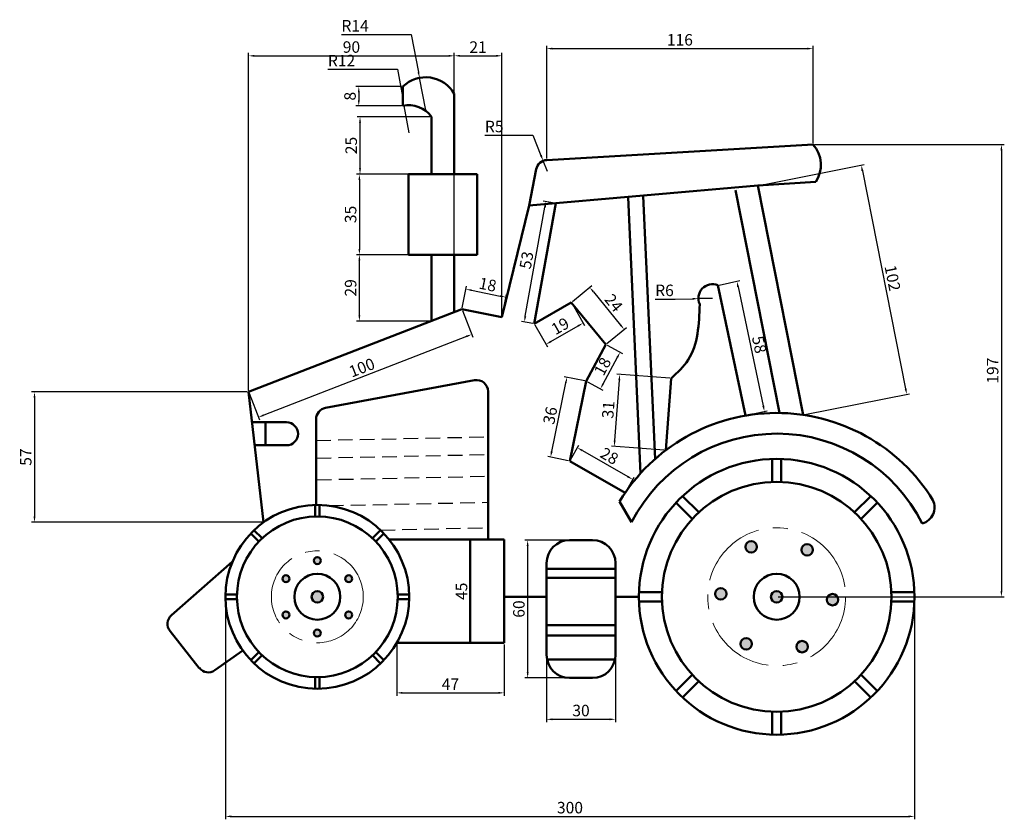
# Model space of a CAD drawing. Units: millimetres. Extents: x 853 to 1282, y 1256 to 1604.
import ezdxf

# ---------------------------------------------------------------- set-up
doc = ezdxf.new("R2010")
doc.units = ezdxf.units.MM
doc.linetypes.add('CENTER', pattern=[50.8, 31.75, -6.35, 6.35, -6.35])
doc.linetypes.add('HIDDEN', pattern=[9.525, 6.35, -3.175])
for name, color, linetype, lineweight in [('M-CNTR', 1, 'CENTER', 18), ('M-DIMS', 2, 'Continuous', 25), ('M-HATC', 8, 'Continuous', 18), ('M-HIDN', 8, 'HIDDEN', 25), ('M-OUTL', 7, 'Continuous', 50)]:
    doc.layers.add(name, color=color, linetype=linetype, lineweight=lineweight)
doc.styles.get("Standard").update_dxf_attribs({"font": 'arial.ttf'})
doc.dimstyles.new('ISO-25', dxfattribs={"dimtxt": 5, "dimasz": 2.5, "dimexe": 1.25, "dimexo": 0.625, "dimtad": 1, "dimtoh": 1, "dimdec": 0, "dimtxsty": 'Standard', "dimcen": 2.5, "dimadec": 0, "dimazin": 0, "dimtfac": 1, "dimtdec": 0, "dimtmove": 0, "dimatfit": 3, "dimfxl": 1, "dimarcsym": 0})

# ---------------------------------------------------------------- blocks, each defined once
blk = doc.blocks.new('*U1')
for p, q in [((-1, 2.5), (-1, -2.5)), ((1, 2.5), (1, -2.5))]:
    blk.add_line(p, q)
blk = doc.blocks.new('*U2')
at = {"layer": 'M-OUTL', "color": 0, "linetype": 'ByBlock', "lineweight": -2, "transparency": 16777216}
blk.add_blockref('*U1', (982.95, 1390.56), dxfattribs=at)
for p, rotation in [((956.43, 1379.58), 45.00000000000001), ((1009.46, 1379.58), 315), ((945.45, 1353.06), 90), ((1020.45, 1353.06), 270), ((956.43, 1326.55), 135), ((1009.46, 1326.55), 225), ((982.95, 1315.56), 180)]:
    blk.add_blockref('*U1', p, dxfattribs=dict(at, rotation=rotation))
blk = doc.blocks.new('*U3')
for p, q in [((-2, -5), (-2, 5)), ((2, -5), (2, 5))]:
    blk.add_line(p, q)
blk = doc.blocks.new('*U4')
at = {"layer": 'M-OUTL', "color": 0, "linetype": 'ByBlock', "lineweight": -2, "transparency": 16777216}
blk.add_blockref('*U3', (1182.95, 1408.06), dxfattribs=at)
for p, rotation in [((1144.05, 1391.96), 45.00000000000001), ((1221.84, 1391.96), 315.0000000000001), ((1127.95, 1353.06), 90), ((1237.95, 1353.06), 270.0000000000001), ((1144.05, 1314.17), 135), ((1221.84, 1314.17), 225), ((1182.95, 1298.06), 180)]:
    blk.add_blockref('*U3', p, dxfattribs=dict(at, rotation=rotation))
blk = doc.blocks.new('*U5')
blk.add_circle((0, 0), 1.5)
blk = doc.blocks.new('*U6')
at = {"layer": 'M-OUTL', "color": 0, "linetype": 'ByBlock', "lineweight": -2, "transparency": 16777216}
blk.add_blockref('*U5', (982.95, 1368.83), dxfattribs=at)
for p, rotation in [((969.3, 1360.95), 60), ((996.6, 1360.94), 300), ((969.3, 1345.19), 120), ((996.59, 1345.18), 240), ((982.94, 1337.3), 180)]:
    blk.add_blockref('*U5', p, dxfattribs=dict(at, rotation=rotation))
blk = doc.blocks.new('*U7')
blk.add_circle((0, 0), 2.5)
blk = doc.blocks.new('*U8')
at = {"layer": 'M-OUTL', "color": 0, "linetype": 'ByBlock', "lineweight": -2, "transparency": 16777216}
for p, rotation in [((1171.87, 1374.78), 59.99999999999999), ((1158.6, 1354.33), 120), ((1207.29, 1351.8), 300), ((1169.68, 1332.61), 180), ((1194.02, 1331.35), 239.9999999999999)]:
    blk.add_blockref('*U7', p, dxfattribs=dict(at, rotation=rotation))
blk.add_blockref('*U7', (1196.21, 1373.52), dxfattribs=at)
blk = doc.blocks.new('*D9')
at = {"layer": 'Defpoints', "color": 0, "lineweight": 100, "transparency": 16777216}
for p in [(942.95, 1353.06), (1242.95, 1353.06), (1242.95, 1257.5)]:
    blk.add_point(p, dxfattribs=at)
at = {"layer": 'M-DIMS', "color": 0, "lineweight": -2, "transparency": 16777216}
for p, q in [((942.95, 1352.44), (942.95, 1256.25)), ((1242.95, 1352.44), (1242.95, 1256.25)), ((945.45, 1257.5), (1240.45, 1257.5))]:
    blk.add_line(p, q, dxfattribs=at)
at = {"layer": 'M-DIMS', "color": 0, "lineweight": 100, "transparency": 16777216}
for points in [[(945.45, 1257.91), (945.45, 1257.08), (942.95, 1257.5)], [(1240.45, 1257.91), (1240.45, 1257.08), (1242.95, 1257.5)]]:
    blk.add_solid(points, dxfattribs=at)
at = {"layer": 'M-DIMS', "color": 0, "transparency": 16777216, "insert": (1092.95, 1260.67), "char_height": 5, "attachment_point": 5}
blk.add_mtext('300', dxfattribs=at)
blk = doc.blocks.new('*D10')
at = {"layer": 'Defpoints', "color": 0, "lineweight": 100, "transparency": 16777216}
for p in [(1198.77, 1549.9), (1182.95, 1353.06), (1280.81, 1353.06)]:
    blk.add_point(p, dxfattribs=at)
at = {"layer": 'M-DIMS', "color": 0, "lineweight": -2, "transparency": 16777216}
for p, q in [((1199.39, 1549.9), (1282.06, 1549.9)), ((1280.81, 1547.4), (1280.81, 1355.56)), ((1183.57, 1353.06), (1282.06, 1353.06))]:
    blk.add_line(p, q, dxfattribs=at)
at = {"layer": 'M-DIMS', "color": 0, "lineweight": 100, "transparency": 16777216}
for points in [[(1280.4, 1547.4), (1281.23, 1547.4), (1280.81, 1549.9)], [(1280.4, 1355.56), (1281.23, 1355.56), (1280.81, 1353.06)]]:
    blk.add_solid(points, dxfattribs=at)
at = {"layer": 'M-DIMS', "color": 0, "transparency": 16777216, "insert": (1277.64, 1451.48), "char_height": 5, "attachment_point": 5, "rotation": 90}
blk.add_mtext('197', dxfattribs=at)
blk = doc.blocks.new('*D11')
at = {"layer": 'Defpoints', "color": 0, "lineweight": 100, "transparency": 16777216}
for p in [(953.02, 1442.19), (859.8, 1385.51), (959.55, 1385.51)]:
    blk.add_point(p, dxfattribs=at)
at = {"layer": 'M-DIMS', "color": 0, "lineweight": -2, "transparency": 16777216}
for p, q in [((952.4, 1442.19), (858.55, 1442.19)), ((859.8, 1439.69), (859.8, 1388.01)), ((958.92, 1385.51), (858.55, 1385.51))]:
    blk.add_line(p, q, dxfattribs=at)
at = {"layer": 'M-DIMS', "color": 0, "lineweight": 100, "transparency": 16777216}
for points in [[(859.39, 1439.69), (860.22, 1439.69), (859.8, 1442.19)], [(859.39, 1388.01), (860.22, 1388.01), (859.8, 1385.51)]]:
    blk.add_solid(points, dxfattribs=at)
at = {"layer": 'M-DIMS', "color": 0, "transparency": 16777216, "insert": (856.64, 1413.85), "char_height": 5, "attachment_point": 5, "rotation": 90}
blk.add_mtext('57', dxfattribs=at)
blk = doc.blocks.new('*D12')
at = {"layer": 'Defpoints', "color": 0, "lineweight": 100, "transparency": 16777216}
for p in [(1042.59, 1588.46), (1042.59, 1476.94), (953.02, 1442.19)]:
    blk.add_point(p, dxfattribs=at)
at = {"layer": 'M-DIMS', "color": 0, "lineweight": -2, "transparency": 16777216}
for p, q in [((953.02, 1442.81), (953.02, 1589.71)), ((955.52, 1588.46), (1040.09, 1588.46)), ((1042.59, 1477.57), (1042.59, 1589.71))]:
    blk.add_line(p, q, dxfattribs=at)
at = {"layer": 'M-DIMS', "color": 0, "lineweight": 100, "transparency": 16777216}
for points in [[(955.52, 1588.87), (955.52, 1588.04), (953.02, 1588.46)], [(1040.09, 1588.87), (1040.09, 1588.04), (1042.59, 1588.46)]]:
    blk.add_solid(points, dxfattribs=at)
at = {"layer": 'M-DIMS', "color": 0, "transparency": 16777216, "insert": (997.8, 1591.64), "char_height": 5, "attachment_point": 5}
blk.add_mtext('90', dxfattribs=at)
blk = doc.blocks.new('*D13')
at = {"layer": 'Defpoints', "color": 0, "lineweight": 100, "transparency": 16777216}
for p in [(1198.77, 1591.61), (1198.77, 1549.9), (1082.84, 1543.13)]:
    blk.add_point(p, dxfattribs=at)
at = {"layer": 'M-DIMS', "color": 0, "lineweight": -2, "transparency": 16777216}
for p, q in [((1082.84, 1543.75), (1082.84, 1592.86)), ((1085.34, 1591.61), (1196.27, 1591.61)), ((1198.77, 1550.52), (1198.77, 1592.86))]:
    blk.add_line(p, q, dxfattribs=at)
at = {"layer": 'M-DIMS', "color": 0, "lineweight": 100, "transparency": 16777216}
for points in [[(1085.34, 1592.03), (1085.34, 1591.19), (1082.84, 1591.61)], [(1196.27, 1592.03), (1196.27, 1591.19), (1198.77, 1591.61)]]:
    blk.add_solid(points, dxfattribs=at)
at = {"layer": 'M-DIMS', "color": 0, "transparency": 16777216, "insert": (1140.8, 1594.79), "char_height": 5, "attachment_point": 5}
blk.add_mtext('116', dxfattribs=at)
blk = doc.blocks.new('*D14')
at = {"layer": 'Defpoints', "color": 0, "lineweight": 100, "transparency": 16777216}
for p in [(1063.29, 1588.49), (1042.59, 1476.94), (1063.29, 1474.7)]:
    blk.add_point(p, dxfattribs=at)
at = {"layer": 'M-DIMS', "color": 0, "lineweight": -2, "transparency": 16777216}
for p, q in [((1042.59, 1477.57), (1042.59, 1589.74)), ((1045.09, 1588.49), (1060.79, 1588.49)), ((1063.29, 1475.32), (1063.29, 1589.74))]:
    blk.add_line(p, q, dxfattribs=at)
at = {"layer": 'M-DIMS', "color": 0, "lineweight": 100, "transparency": 16777216}
for points in [[(1045.09, 1588.9), (1045.09, 1588.07), (1042.59, 1588.49)], [(1060.79, 1588.9), (1060.79, 1588.07), (1063.29, 1588.49)]]:
    blk.add_solid(points, dxfattribs=at)
at = {"layer": 'M-DIMS', "color": 0, "transparency": 16777216, "insert": (1052.94, 1591.62), "char_height": 5, "attachment_point": 5}
blk.add_mtext('21', dxfattribs=at)
blk = doc.blocks.new('*D15')
at = {"layer": 'Defpoints', "color": 0, "lineweight": 100, "transparency": 16777216}
for p in [(1082.76, 1347.74), (1112.76, 1347.74), (1112.76, 1299.75)]:
    blk.add_point(p, dxfattribs=at)
at = {"layer": 'M-DIMS', "color": 0, "lineweight": -2, "transparency": 16777216}
for p, q in [((1082.76, 1347.12), (1082.76, 1298.5)), ((1112.76, 1347.12), (1112.76, 1298.5)), ((1085.26, 1299.75), (1110.26, 1299.75))]:
    blk.add_line(p, q, dxfattribs=at)
at = {"layer": 'M-DIMS', "color": 0, "lineweight": 100, "transparency": 16777216}
for points in [[(1085.26, 1300.16), (1085.26, 1299.33), (1082.76, 1299.75)], [(1110.26, 1300.16), (1110.26, 1299.33), (1112.76, 1299.75)]]:
    blk.add_solid(points, dxfattribs=at)
at = {"layer": 'M-DIMS', "color": 0, "transparency": 16777216, "insert": (1097.76, 1302.93), "char_height": 5, "attachment_point": 5}
blk.add_mtext('30', dxfattribs=at)
blk = doc.blocks.new('*D16')
at = {"layer": 'Defpoints', "color": 0, "lineweight": 100, "transparency": 16777216}
for p in [(1097.76, 1377.74), (1074.52, 1317.74), (1097.76, 1317.74)]:
    blk.add_point(p, dxfattribs=at)
at = {"layer": 'M-DIMS', "color": 0, "lineweight": -2, "transparency": 16777216}
for p, q in [((1097.14, 1377.74), (1073.27, 1377.74)), ((1074.52, 1375.24), (1074.52, 1320.24)), ((1097.14, 1317.74), (1073.27, 1317.74))]:
    blk.add_line(p, q, dxfattribs=at)
at = {"layer": 'M-DIMS', "color": 0, "lineweight": 100, "transparency": 16777216}
for points in [[(1074.11, 1375.24), (1074.94, 1375.24), (1074.52, 1377.74)], [(1074.11, 1320.24), (1074.94, 1320.24), (1074.52, 1317.74)]]:
    blk.add_solid(points, dxfattribs=at)
at = {"layer": 'M-DIMS', "color": 0, "transparency": 16777216, "insert": (1071.35, 1347.74), "char_height": 5, "attachment_point": 5, "rotation": 90}
blk.add_mtext('60', dxfattribs=at)
blk = doc.blocks.new('*D17')
at = {"layer": 'Defpoints', "color": 0, "lineweight": 100, "transparency": 16777216}
for p in [(1049.53, 1377.96), (1049.53, 1332.96), (1049.53, 1332.96)]:
    blk.add_point(p, dxfattribs=at)
at = {"layer": 'M-DIMS', "color": 0, "lineweight": -2, "transparency": 16777216}
for p, q in [((1050.16, 1377.96), (1050.78, 1377.96)), ((1049.53, 1375.46), (1049.53, 1335.46)), ((1050.16, 1332.96), (1050.78, 1332.96))]:
    blk.add_line(p, q, dxfattribs=at)
at = {"layer": 'M-DIMS', "color": 0, "lineweight": 100, "transparency": 16777216}
for points in [[(1049.12, 1375.46), (1049.95, 1375.46), (1049.53, 1377.96)], [(1049.12, 1335.46), (1049.95, 1335.46), (1049.53, 1332.96)]]:
    blk.add_solid(points, dxfattribs=at)
at = {"layer": 'M-DIMS', "color": 0, "transparency": 16777216, "insert": (1046.37, 1355.46), "char_height": 5, "attachment_point": 5, "rotation": 90}
blk.add_mtext('45', dxfattribs=at)
blk = doc.blocks.new('*D18')
at = {"layer": 'Defpoints', "color": 0, "lineweight": 100, "transparency": 16777216}
for p in [(1017.53, 1332.96), (1064.25, 1332.96), (1064.25, 1311.26)]:
    blk.add_point(p, dxfattribs=at)
at = {"layer": 'M-DIMS', "color": 0, "lineweight": -2, "transparency": 16777216}
for p, q in [((1017.53, 1332.33), (1017.53, 1310.01)), ((1064.25, 1332.33), (1064.25, 1310.01)), ((1020.03, 1311.26), (1061.75, 1311.26))]:
    blk.add_line(p, q, dxfattribs=at)
at = {"layer": 'M-DIMS', "color": 0, "lineweight": 100, "transparency": 16777216}
for points in [[(1020.03, 1311.68), (1020.03, 1310.84), (1017.53, 1311.26)], [(1061.75, 1311.68), (1061.75, 1310.84), (1064.25, 1311.26)]]:
    blk.add_solid(points, dxfattribs=at)
at = {"layer": 'M-DIMS', "color": 0, "transparency": 16777216, "insert": (1040.89, 1314.38), "char_height": 5, "attachment_point": 5}
blk.add_mtext('47', dxfattribs=at)
blk = doc.blocks.new('*D19')
at = {"layer": 'Defpoints', "color": 0, "lineweight": 100, "transparency": 16777216}
for p in [(1174.77, 1531.97), (1239.58, 1441.15), (1194.55, 1432.22)]:
    blk.add_point(p, dxfattribs=at)
at = {"layer": 'M-DIMS', "color": 0, "lineweight": -2, "transparency": 16777216}
for p, q in [((1175.38, 1532.09), (1221.02, 1541.14)), ((1220.28, 1538.45), (1239.09, 1443.6)), ((1195.16, 1432.34), (1240.8, 1441.39))]:
    blk.add_line(p, q, dxfattribs=at)
at = {"layer": 'M-DIMS', "color": 0, "lineweight": 100, "transparency": 16777216}
for points in [[(1220.69, 1538.53), (1219.87, 1538.37), (1219.8, 1540.9)], [(1239.5, 1443.68), (1238.68, 1443.52), (1239.58, 1441.15)]]:
    blk.add_solid(points, dxfattribs=at)
at = {"layer": 'M-DIMS', "color": 0, "transparency": 16777216, "insert": (1232.8, 1491.64), "char_height": 5, "attachment_point": 5, "rotation": 281.2154}
blk.add_mtext('102', dxfattribs=at)
blk = doc.blocks.new('*D20')
at = {"layer": 'Defpoints', "color": 0, "lineweight": 100, "transparency": 16777216}
for p in [(1157.31, 1488.61), (1169.34, 1431.9), (1177.65, 1433.66)]:
    blk.add_point(p, dxfattribs=at)
at = {"layer": 'M-DIMS', "color": 0, "lineweight": -2, "transparency": 16777216}
for p, q in [((1157.92, 1488.74), (1166.84, 1490.63)), ((1166.14, 1487.93), (1177.13, 1436.11)), ((1169.95, 1432.03), (1178.87, 1433.92))]:
    blk.add_line(p, q, dxfattribs=at)
at = {"layer": 'M-DIMS', "color": 0, "lineweight": 100, "transparency": 16777216}
for points in [[(1166.55, 1488.02), (1165.73, 1487.84), (1165.62, 1490.37)], [(1177.54, 1436.19), (1176.72, 1436.02), (1177.65, 1433.66)]]:
    blk.add_solid(points, dxfattribs=at)
at = {"layer": 'M-DIMS', "color": 0, "transparency": 16777216, "insert": (1174.74, 1462.68), "char_height": 5, "attachment_point": 5, "rotation": 281.9736}
blk.add_mtext('58', dxfattribs=at)
blk = doc.blocks.new('*D21')
at = {"layer": 'Defpoints', "color": 0, "lineweight": 100, "transparency": 16777216}
for p in [(1137.03, 1448.09), (1112.22, 1418.55), (1134.64, 1416.83)]:
    blk.add_point(p, dxfattribs=at)
at = {"layer": 'M-DIMS', "color": 0, "lineweight": -2, "transparency": 16777216}
for p, q in [((1136.41, 1448.13), (1113.37, 1449.9)), ((1114.42, 1447.31), (1112.41, 1421.04)), ((1134.02, 1416.88), (1110.98, 1418.65))]:
    blk.add_line(p, q, dxfattribs=at)
at = {"layer": 'M-DIMS', "color": 0, "lineweight": 100, "transparency": 16777216}
for points in [[(1114.01, 1447.34), (1114.84, 1447.28), (1114.61, 1449.8)], [(1112, 1421.07), (1112.83, 1421.01), (1112.22, 1418.55)]]:
    blk.add_solid(points, dxfattribs=at)
at = {"layer": 'M-DIMS', "color": 0, "transparency": 16777216, "insert": (1110.25, 1434.42), "char_height": 5, "attachment_point": 5, "rotation": 85.6221}
blk.add_mtext('31', dxfattribs=at)
blk = doc.blocks.new('*D22')
at = {"layer": 'Defpoints', "color": 0, "lineweight": 100, "transparency": 16777216}
for p in [(1092.82, 1412.09), (1120.29, 1404.11), (1116.94, 1398.26)]:
    blk.add_point(p, dxfattribs=at)
at = {"layer": 'M-DIMS', "color": 0, "lineweight": -2, "transparency": 16777216}
for p, q in [((1093.13, 1412.64), (1096.8, 1419.02)), ((1098.35, 1416.7), (1118.12, 1405.35)), ((1117.25, 1398.8), (1120.91, 1405.19))]:
    blk.add_line(p, q, dxfattribs=at)
at = {"layer": 'M-DIMS', "color": 0, "lineweight": 100, "transparency": 16777216}
for points in [[(1098.55, 1417.06), (1098.14, 1416.33), (1096.18, 1417.94)], [(1118.33, 1405.71), (1117.91, 1404.99), (1120.29, 1404.11)]]:
    blk.add_solid(points, dxfattribs=at)
at = {"layer": 'M-DIMS', "color": 0, "transparency": 16777216, "insert": (1109.81, 1413.78), "char_height": 5, "attachment_point": 5, "rotation": 330.159}
blk.add_mtext('28', dxfattribs=at)
blk = doc.blocks.new('*D23')
at = {"layer": 'Defpoints', "color": 0, "lineweight": 100, "transparency": 16777216}
for p in [(1091.65, 1448.59), (1099.98, 1446.87), (1092.82, 1412.09)]:
    blk.add_point(p, dxfattribs=at)
at = {"layer": 'M-DIMS', "color": 0, "lineweight": -2, "transparency": 16777216}
for p, q in [((1085, 1416.26), (1091.14, 1446.14)), ((1099.36, 1447), (1090.42, 1448.84)), ((1092.21, 1412.22), (1083.27, 1414.06))]:
    blk.add_line(p, q, dxfattribs=at)
at = {"layer": 'M-DIMS', "color": 0, "lineweight": 100, "transparency": 16777216}
for points in [[(1090.74, 1446.22), (1091.55, 1446.05), (1091.65, 1448.59)], [(1084.59, 1416.34), (1085.41, 1416.17), (1084.5, 1413.81)]]:
    blk.add_solid(points, dxfattribs=at)
at = {"layer": 'M-DIMS', "color": 0, "transparency": 16777216, "insert": (1084.96, 1431.84), "char_height": 5, "attachment_point": 5, "rotation": 78.3786}
blk.add_mtext('36', dxfattribs=at)
blk = doc.blocks.new('*D24')
at = {"layer": 'Defpoints', "color": 0, "lineweight": 100, "transparency": 16777216}
for p in [(1108.56, 1462.83), (1114.78, 1459.49), (1099.98, 1446.87)]:
    blk.add_point(p, dxfattribs=at)
at = {"layer": 'M-DIMS', "color": 0, "lineweight": -2, "transparency": 16777216}
for p, q in [((1109.11, 1462.54), (1115.89, 1458.89)), ((1107.39, 1445.73), (1113.6, 1457.28)), ((1100.53, 1446.58), (1107.3, 1442.93))]:
    blk.add_line(p, q, dxfattribs=at)
at = {"layer": 'M-DIMS', "color": 0, "lineweight": 100, "transparency": 16777216}
for points in [[(1113.23, 1457.48), (1113.97, 1457.09), (1114.78, 1459.49)], [(1107.02, 1445.92), (1107.75, 1445.53), (1106.2, 1443.53)]]:
    blk.add_solid(points, dxfattribs=at)
at = {"layer": 'M-DIMS', "color": 0, "transparency": 16777216, "insert": (1107.69, 1453.01), "char_height": 5, "attachment_point": 5, "rotation": 61.7294}
blk.add_mtext('18', dxfattribs=at)
blk = doc.blocks.new('*D25')
at = {"layer": 'Defpoints', "color": 0, "lineweight": 100, "transparency": 16777216}
for p in [(1093.54, 1481.18), (1116.57, 1469.4), (1108.56, 1462.83)]:
    blk.add_point(p, dxfattribs=at)
at = {"layer": 'M-DIMS', "color": 0, "lineweight": -2, "transparency": 16777216}
for p, q in [((1094.02, 1481.57), (1102.52, 1488.53)), ((1103.14, 1485.8), (1114.99, 1471.33)), ((1109.04, 1463.23), (1117.54, 1470.19))]:
    blk.add_line(p, q, dxfattribs=at)
at = {"layer": 'M-DIMS', "color": 0, "lineweight": 100, "transparency": 16777216}
for points in [[(1103.46, 1486.07), (1102.81, 1485.54), (1101.55, 1487.74)], [(1115.31, 1471.59), (1114.67, 1471.07), (1116.57, 1469.4)]]:
    blk.add_solid(points, dxfattribs=at)
at = {"layer": 'M-DIMS', "color": 0, "transparency": 16777216, "insert": (1111.49, 1480.55), "char_height": 5, "attachment_point": 5, "rotation": 309.3139}
blk.add_mtext('24', dxfattribs=at)
blk = doc.blocks.new('*D26')
at = {"layer": 'Defpoints', "color": 0, "lineweight": 100, "transparency": 16777216}
for p in [(1093.54, 1481.18), (1077.33, 1471.89), (1098.69, 1472.19)]:
    blk.add_point(p, dxfattribs=at)
at = {"layer": 'M-DIMS', "color": 0, "lineweight": -2, "transparency": 16777216}
for p, q in [((1093.85, 1480.63), (1099.31, 1471.11)), ((1077.64, 1471.34), (1083.1, 1461.82)), ((1084.64, 1464.15), (1096.52, 1470.95))]:
    blk.add_line(p, q, dxfattribs=at)
at = {"layer": 'M-DIMS', "color": 0, "lineweight": 100, "transparency": 16777216}
for points in [[(1096.31, 1471.31), (1096.72, 1470.59), (1098.69, 1472.19)], [(1084.44, 1464.51), (1084.85, 1463.78), (1082.47, 1462.9)]]:
    blk.add_solid(points, dxfattribs=at)
at = {"layer": 'M-DIMS', "color": 0, "transparency": 16777216, "insert": (1089, 1470.3), "char_height": 5, "attachment_point": 5, "rotation": 29.8139}
blk.add_mtext('19', dxfattribs=at)
blk = doc.blocks.new('*D27')
at = {"layer": 'Defpoints', "color": 0, "lineweight": 100, "transparency": 16777216}
for p in [(1082.52, 1525.06), (1086.78, 1524.29), (1077.33, 1471.89)]:
    blk.add_point(p, dxfattribs=at)
at = {"layer": 'M-DIMS', "color": 0, "lineweight": -2, "transparency": 16777216}
for p, q in [((1073.51, 1475.12), (1082.07, 1522.6)), ((1086.17, 1524.4), (1081.29, 1525.28)), ((1076.71, 1472), (1071.83, 1472.88))]:
    blk.add_line(p, q, dxfattribs=at)
at = {"layer": 'M-DIMS', "color": 0, "lineweight": 100, "transparency": 16777216}
for points in [[(1081.66, 1522.67), (1082.48, 1522.52), (1082.52, 1525.06)], [(1073.1, 1475.19), (1073.92, 1475.04), (1073.06, 1472.65)]]:
    blk.add_solid(points, dxfattribs=at)
at = {"layer": 'M-DIMS', "color": 0, "transparency": 16777216, "insert": (1074.66, 1499.42), "char_height": 5, "attachment_point": 5, "rotation": 79.7728}
blk.add_mtext('53', dxfattribs=at)
blk = doc.blocks.new('*D28')
at = {"layer": 'Defpoints', "color": 0, "lineweight": 100, "transparency": 16777216}
for p in [(1065.06, 1483.42), (1045.92, 1478.23), (1063.29, 1474.7)]:
    blk.add_point(p, dxfattribs=at)
at = {"layer": 'M-DIMS', "color": 0, "lineweight": -2, "transparency": 16777216}
for p, q in [((1046.04, 1478.84), (1047.94, 1488.18)), ((1050.14, 1486.46), (1062.61, 1483.92)), ((1063.41, 1475.31), (1065.31, 1484.65))]:
    blk.add_line(p, q, dxfattribs=at)
at = {"layer": 'M-DIMS', "color": 0, "lineweight": 100, "transparency": 16777216}
for points in [[(1050.23, 1486.87), (1050.06, 1486.05), (1047.69, 1486.96)], [(1062.69, 1484.33), (1062.53, 1483.51), (1065.06, 1483.42)]]:
    blk.add_solid(points, dxfattribs=at)
at = {"layer": 'M-DIMS', "color": 0, "transparency": 16777216, "insert": (1057.01, 1488.3), "char_height": 5, "attachment_point": 5, "rotation": 348.5016}
blk.add_mtext('18', dxfattribs=at)
blk = doc.blocks.new('*D29')
at = {"layer": 'Defpoints', "color": 0, "lineweight": 100, "transparency": 16777216}
for p in [(1045.92, 1478.23), (953.02, 1442.19), (957.28, 1431.21)]:
    blk.add_point(p, dxfattribs=at)
at = {"layer": 'M-DIMS', "color": 0, "lineweight": -2, "transparency": 16777216}
for p, q in [((1046.14, 1477.65), (1050.63, 1466.08)), ((1047.85, 1466.34), (959.61, 1432.11)), ((953.25, 1441.61), (957.73, 1430.04))]:
    blk.add_line(p, q, dxfattribs=at)
at = {"layer": 'M-DIMS', "color": 0, "lineweight": 100, "transparency": 16777216}
for points in [[(1047.7, 1466.73), (1048, 1465.96), (1050.18, 1467.25)], [(959.46, 1432.5), (959.76, 1431.72), (957.28, 1431.21)]]:
    blk.add_solid(points, dxfattribs=at)
at = {"layer": 'M-DIMS', "color": 0, "transparency": 16777216, "insert": (1002.58, 1452.19), "char_height": 5, "attachment_point": 5, "rotation": 21.2055}
blk.add_mtext('100', dxfattribs=at)
blk = doc.blocks.new('*D30')
at = {"layer": 'Defpoints', "color": 0, "lineweight": 100, "transparency": 16777216}
for p in [(1001.26, 1501.94), (1032.59, 1501.94), (1032.59, 1473.06)]:
    blk.add_point(p, dxfattribs=at)
at = {"layer": 'M-DIMS', "color": 0, "lineweight": -2, "transparency": 16777216}
for p, q in [((1031.96, 1501.94), (1000.01, 1501.94)), ((1001.26, 1475.56), (1001.26, 1499.44)), ((1031.96, 1473.06), (1000.01, 1473.06))]:
    blk.add_line(p, q, dxfattribs=at)
at = {"layer": 'M-DIMS', "color": 0, "lineweight": 100, "transparency": 16777216}
for points in [[(1000.85, 1499.44), (1001.68, 1499.44), (1001.26, 1501.94)], [(1000.85, 1475.56), (1001.68, 1475.56), (1001.26, 1473.06)]]:
    blk.add_solid(points, dxfattribs=at)
at = {"layer": 'M-DIMS', "color": 0, "transparency": 16777216, "insert": (998.09, 1487.5), "char_height": 5, "attachment_point": 5, "rotation": 90}
blk.add_mtext('29', dxfattribs=at)
blk = doc.blocks.new('*D31')
at = {"layer": 'Defpoints', "color": 0, "lineweight": 100, "transparency": 16777216}
for p in [(1022.59, 1536.94), (1001.26, 1501.94), (1022.59, 1501.94)]:
    blk.add_point(p, dxfattribs=at)
at = {"layer": 'M-DIMS', "color": 0, "lineweight": -2, "transparency": 16777216}
for p, q in [((1021.96, 1536.94), (1000.01, 1536.94)), ((1001.26, 1534.44), (1001.26, 1504.44)), ((1021.96, 1501.94), (1000.01, 1501.94))]:
    blk.add_line(p, q, dxfattribs=at)
at = {"layer": 'M-DIMS', "color": 0, "lineweight": 100, "transparency": 16777216}
for points in [[(1000.85, 1534.44), (1001.68, 1534.44), (1001.26, 1536.94)], [(1000.85, 1504.44), (1001.68, 1504.44), (1001.26, 1501.94)]]:
    blk.add_solid(points, dxfattribs=at)
at = {"layer": 'M-DIMS', "color": 0, "transparency": 16777216, "insert": (998.09, 1519.44), "char_height": 5, "attachment_point": 5, "rotation": 90}
blk.add_mtext('35', dxfattribs=at)
blk = doc.blocks.new('*D32')
at = {"layer": 'Defpoints', "color": 0, "lineweight": 100, "transparency": 16777216}
for p in [(1001.53, 1561.94), (1032.59, 1561.94), (1032.59, 1536.94)]:
    blk.add_point(p, dxfattribs=at)
at = {"layer": 'M-DIMS', "color": 0, "lineweight": -2, "transparency": 16777216}
for p, q in [((1031.96, 1561.94), (1000.28, 1561.94)), ((1001.53, 1539.44), (1001.53, 1559.44)), ((1031.96, 1536.94), (1000.28, 1536.94))]:
    blk.add_line(p, q, dxfattribs=at)
at = {"layer": 'M-DIMS', "color": 0, "lineweight": 100, "transparency": 16777216}
for points in [[(1001.12, 1559.44), (1001.95, 1559.44), (1001.53, 1561.94)], [(1001.12, 1539.44), (1001.95, 1539.44), (1001.53, 1536.94)]]:
    blk.add_solid(points, dxfattribs=at)
at = {"layer": 'M-DIMS', "color": 0, "transparency": 16777216, "insert": (998.35, 1549.44), "char_height": 5, "attachment_point": 5, "rotation": 90}
blk.add_mtext('25', dxfattribs=at)
blk = doc.blocks.new('*D33')
at = {"layer": 'Defpoints', "color": 0, "lineweight": 100, "transparency": 16777216}
for p in [(1020.18, 1575.12), (1001, 1566.65), (1020.18, 1566.65)]:
    blk.add_point(p, dxfattribs=at)
at = {"layer": 'M-DIMS', "color": 0, "lineweight": -2, "transparency": 16777216}
for p, q in [((1019.56, 1575.12), (999.75, 1575.12)), ((1001, 1572.62), (1001, 1569.15)), ((1019.56, 1566.65), (999.75, 1566.65))]:
    blk.add_line(p, q, dxfattribs=at)
at = {"layer": 'M-DIMS', "color": 0, "lineweight": 100, "transparency": 16777216}
for points in [[(1000.58, 1572.62), (1001.41, 1572.62), (1001, 1575.12)], [(1000.58, 1569.15), (1001.41, 1569.15), (1001, 1566.65)]]:
    blk.add_solid(points, dxfattribs=at)
at = {"layer": 'M-DIMS', "color": 0, "transparency": 16777216, "insert": (997.82, 1570.89), "char_height": 5, "attachment_point": 5, "rotation": 90}
blk.add_mtext('8', dxfattribs=at)
blk = doc.blocks.new('*D34')
at = {"layer": 'Defpoints', "color": 0, "lineweight": 100, "transparency": 16777216}
for p in [(1027.46, 1578.88), (1030.14, 1564.76)]:
    blk.add_point(p, dxfattribs=at)
at = {"layer": 'M-DIMS', "color": 0, "lineweight": -2, "transparency": 16777216}
for p, q in [((993.43, 1597.77), (1023.87, 1597.77)), ((1023.87, 1597.77), (1026.99, 1581.34)), ((1030.14, 1564.76), (1027.46, 1578.88))]:
    blk.add_line(p, q, dxfattribs=at)
at = {"layer": 'M-DIMS', "color": 0, "lineweight": 100, "transparency": 16777216}
blk.add_solid([(1027.4, 1581.41), (1026.58, 1581.26), (1027.46, 1578.88)], dxfattribs=at)
at = {"layer": 'M-DIMS', "color": 0, "transparency": 16777216, "insert": (999.39, 1600.9), "char_height": 5, "attachment_point": 5}
blk.add_mtext('R14', dxfattribs=at)
blk = doc.blocks.new('*D35')
at = {"layer": 'Defpoints', "color": 0, "lineweight": 100, "transparency": 16777216}
for p in [(1020.75, 1566.77), (1022.87, 1555.03)]:
    blk.add_point(p, dxfattribs=at)
at = {"layer": 'M-DIMS', "color": 0, "lineweight": -2, "transparency": 16777216}
for p, q in [((987.53, 1582.62), (1017.89, 1582.62)), ((1017.89, 1582.62), (1020.31, 1569.23)), ((1022.87, 1555.03), (1020.75, 1566.77))]:
    blk.add_line(p, q, dxfattribs=at)
at = {"layer": 'M-DIMS', "color": 0, "lineweight": 100, "transparency": 16777216}
blk.add_solid([(1020.72, 1569.3), (1019.9, 1569.16), (1020.75, 1566.77)], dxfattribs=at)
at = {"layer": 'M-DIMS', "color": 0, "transparency": 16777216, "insert": (993.48, 1585.75), "char_height": 5, "attachment_point": 5}
blk.add_mtext('R12', dxfattribs=at)
blk = doc.blocks.new('*D36')
at = {"layer": 'Defpoints', "color": 0, "lineweight": 100, "transparency": 16777216}
for p in [(1081.27, 1542.78), (1083.14, 1538.14)]:
    blk.add_point(p, dxfattribs=at)
at = {"layer": 'M-DIMS', "color": 0, "lineweight": -2, "transparency": 16777216}
for p, q in [((1055.91, 1553.89), (1076.78, 1553.89)), ((1076.78, 1553.89), (1080.33, 1545.09)), ((1083.14, 1538.14), (1081.27, 1542.78))]:
    blk.add_line(p, q, dxfattribs=at)
at = {"layer": 'M-DIMS', "color": 0, "lineweight": 100, "transparency": 16777216}
blk.add_solid([(1080.72, 1545.25), (1079.94, 1544.94), (1081.27, 1542.78)], dxfattribs=at)
at = {"layer": 'M-DIMS', "color": 0, "transparency": 16777216, "insert": (1059.96, 1557.06), "char_height": 5, "attachment_point": 5}
blk.add_mtext('R5', dxfattribs=at)
blk = doc.blocks.new('*D37')
at = {"layer": 'Defpoints', "color": 0, "lineweight": 100, "transparency": 16777216}
for p in [(1148.87, 1482.8), (1155, 1482.94)]:
    blk.add_point(p, dxfattribs=at)
at = {"layer": 'M-DIMS', "color": 0, "lineweight": -2, "transparency": 16777216}
for p, q in [((1130.08, 1482.58), (1138.77, 1482.58)), ((1138.77, 1482.58), (1146.37, 1482.75)), ((1155, 1482.94), (1148.87, 1482.8))]:
    blk.add_line(p, q, dxfattribs=at)
at = {"layer": 'M-DIMS', "color": 0, "lineweight": 100, "transparency": 16777216}
blk.add_solid([(1146.36, 1483.16), (1146.38, 1482.33), (1148.87, 1482.8)], dxfattribs=at)
at = {"layer": 'M-DIMS', "color": 0, "transparency": 16777216, "insert": (1134.11, 1485.76), "char_height": 5, "attachment_point": 5}
blk.add_mtext('R6', dxfattribs=at)
blk = doc.blocks.new('WHEEL-HUB')
for radius in [10, 2.5]:
    blk.add_circle((982.95, 1353.06), radius)

msp = doc.modelspace()

# ---------------------------------------------------------------- hatches: boundary and pattern name
at = {"layer": 'M-HATC'}
h = msp.add_hatch(color=256, dxfattribs=at)
h.set_gradient(color2=(0, 0, 0), tint=1)
h.paths.add_polyline_path([(970.8, 1360.95, 1), (967.8, 1360.95, 1)])
h.paths.add_polyline_path([(984.45, 1368.83, 1), (981.45, 1368.83, 1)])
h.paths.add_polyline_path([(998.1, 1360.94, 1), (995.1, 1360.94, 1)])
h.paths.add_polyline_path([(995.09, 1345.18, 1), (998.09, 1345.18, 1)])
h.paths.add_polyline_path([(981.44, 1337.3, 1), (984.44, 1337.3, 1)])
h.paths.add_polyline_path([(970.8, 1345.19, 1), (967.8, 1345.19, 1)])
h.paths.add_polyline_path([(985.45, 1353.06, 1), (980.45, 1353.06, 1)])
h.paths.add_polyline_path([(1156.1, 1354.33, 1), (1161.1, 1354.33, 1)])
h.paths.add_polyline_path([(1167.18, 1332.61, 1), (1172.18, 1332.61, 1)])
h.paths.add_polyline_path([(1196.52, 1331.35, 1), (1191.52, 1331.35, 1)])
h.paths.add_polyline_path([(1209.79, 1351.8, 1), (1204.79, 1351.8, 1)])
h.paths.add_polyline_path([(1198.71, 1373.52, 1), (1193.71, 1373.52, 1)])
h.paths.add_polyline_path([(1174.37, 1374.78, 1), (1169.37, 1374.78, 1)])
h.paths.add_polyline_path([(1185.45, 1353.06, 1), (1180.45, 1353.06, 1)])

# ---------------------------------------------------------------- linework, layer by layer
at = {"layer": 'M-CNTR'}
for centre, radius in [((1182.95, 1353.06), 30), ((982.95, 1353.06), 20)]:
    msp.add_circle(centre, radius, dxfattribs=at)
at = {"layer": 'M-HIDN'}
for p, q in [((982.43, 1421.12), (1057.26, 1422.69)), ((982.6, 1413.43), (1057.26, 1414.99)), ((982.79, 1403.98), (1057.26, 1405.54)), ((988.02, 1392.74), (1057.26, 1394.19)), ((1010.43, 1382.12), (1057.26, 1383.11))]:
    msp.add_line(p, q, dxfattribs=at)
at = {"layer": 'M-OUTL'}
for p, q in [((1020.18, 1575.12), (1020.18, 1566.65)), ((1042.59, 1536.94), (1042.59, 1571.94)), ((1032.59, 1536.94), (1032.59, 1561.94)), ((1082.84, 1543.13), (1198.77, 1549.9)), ((1075.15, 1523.27), (1078.23, 1539.09)), ((1022.59, 1501.94), (1022.59, 1536.94)), ((1022.59, 1536.94), (1042.59, 1536.94)), ((1042.59, 1536.94), (1052.59, 1536.94)), ((1052.59, 1536.94), (1052.59, 1501.94)), ((1174.77, 1531.97), (1075.15, 1523.27)), ((1174.77, 1531.97), (1199.96, 1533.6)), ((1194.55, 1432.22), (1174.77, 1531.97)), ((1118.23, 1527.03), (1123.62, 1406.73)), ((1124.88, 1527.33), (1130, 1413.04)), ((1184.19, 1433.06), (1164.96, 1530.03)), ((1075.15, 1523.27), (1063.29, 1474.7)), ((1086.78, 1524.29), (1077.33, 1471.89)), ((1032.59, 1501.94), (1022.59, 1501.94)), ((1042.59, 1501.94), (1032.59, 1501.94)), ((1032.59, 1501.94), (1032.59, 1473.06)), ((1042.59, 1476.94), (1042.59, 1501.94)), ((1052.59, 1501.94), (1042.59, 1501.94)), ((1169.34, 1431.9), (1157.31, 1488.61)), ((1157.31, 1488.61), (1157.31, 1488.61)), ((1077.33, 1471.89), (1093.54, 1481.18)), ((1093.54, 1481.18), (1108.56, 1462.83)), ((1045.92, 1478.23), (953.02, 1442.19)), ((1063.29, 1474.7), (1045.92, 1478.23)), ((1108.56, 1462.83), (1099.98, 1446.87)), ((1051.34, 1447.32), (986.52, 1435.3)), ((1099.98, 1446.87), (1092.82, 1412.09)), ((1134.64, 1416.83), (1137.03, 1448.09)), ((953.02, 1442.19), (959.55, 1385.51)), ((1057.26, 1377.96), (1057.26, 1442.4)), ((954.54, 1428.99), (969.54, 1428.99)), ((960.4, 1428.99), (960.4, 1418.99)), ((982.43, 1430.38), (982.43, 1393.06)), ((969.54, 1418.99), (955.69, 1418.99)), ((1092.82, 1412.09), (1116.94, 1398.26)), ((1114.57, 1394.6), (1119.8, 1385.52)), ((1251, 1395.12), (1251, 1395.12)), ((1246.35, 1385.02), (1246.35, 1385.02)), ((1014.25, 1377.96), (1064.25, 1377.96)), ((1049.53, 1377.96), (1049.53, 1332.96)), ((1064.25, 1377.96), (1064.25, 1332.96)), ((1092.76, 1377.74), (1102.76, 1377.74)), ((945.94, 1368.25), (919.44, 1345.03)), ((1082.76, 1327.74), (1082.76, 1367.74)), ((1112.76, 1367.74), (1112.76, 1327.74)), ((1082.76, 1365.23), (1112.76, 1365.23)), ((1082.76, 1361.37), (1112.76, 1361.37)), ((1064.25, 1353.06), (1082.76, 1353.06)), ((1112.76, 1353.06), (1122.95, 1353.06)), ((918.82, 1338.16), (931.57, 1322.08)), ((1082.76, 1340.73), (1112.76, 1340.73)), ((1082.76, 1336.23), (1112.76, 1336.23)), ((938.36, 1321.1), (950.52, 1329.65)), ((1064.25, 1332.96), (1017.53, 1332.96)), ((1082.97, 1325.72), (1112.56, 1325.72)), ((1102.76, 1317.74), (1092.76, 1317.74))]:
    msp.add_line(p, q, dxfattribs=at)
for centre, radius in [((1182.95, 1353.06), 60), ((1182.95, 1353.06), 50), ((982.95, 1353.06), 40), ((982.95, 1353.06), 35)]:
    msp.add_circle(centre, radius, dxfattribs=at)
for centre, radius, start, end in [((1030.14, 1564.76), 14.37, 29.9667, 133.8769), ((1022.87, 1555.03), 11.93, 35.4016, 103.0032), ((1189.01, 1540.99), 13.21, 325.9691, 42.3887), ((1083.14, 1538.14), 5, 93.3416, 168.9902), ((1155, 1482.94), 6.13, 67.8053, 205.0822), ((1052.26, 1442.4), 5, 0, 100.5037), ((987.43, 1430.38), 5, 100.5037, 180), ((1182.95, 1353.06), 80, 31.7131, 148.7259), ((969.54, 1423.99), 5, 270, 90), ((1182.95, 1353.06), 71, 26.7481, 152.8032), ((1244.45, 1392.02), 7.25, 285.209, 25.317), ((1092.76, 1367.74), 10, 90, 180), ((1102.76, 1367.74), 10, 0, 90), ((922.73, 1341.27), 5, 131.2308, 218.4214), ((1092.76, 1327.74), 10, 180, 270), ((1102.76, 1327.74), 10, 270, 0), ((935.49, 1325.19), 5, 218.4214, 305.1196)]:
    msp.add_arc(centre, radius, start, end, dxfattribs=at)
msp.add_open_spline([(1137.03, 1448.09), (1139.76, 1450.65), (1148.65, 1458.97), (1149.12, 1471.6), (1149.45, 1480.34)], degree=3, knots=[0, 0, 0, 0, 10.966149, 35.645273, 35.645273, 35.645273, 35.645273], dxfattribs=at)

# ---------------------------------------------------------------- block references
for name, p in [('*U4', (0, 0)), ('*U2', (0, 0)), ('*U8', (0, 0)), ('*U6', (0, 0)), ('WHEEL-HUB', (0, 0)), ('WHEEL-HUB', (200, 0))]:
    msp.add_blockref(name, p, dxfattribs=at)

# ---------------------------------------------------------------- dimensions: what is measured, and where the dimension line sits
at = {"layer": 'M-DIMS'}
for center, mpoint, picture, middle in [((1030.14, 1564.76), (1027.46, 1578.88), '*D34', (999.39, 1597.77)), ((1022.87, 1555.03), (1020.75, 1566.77), '*D35', (993.48, 1582.62)), ((1083.14, 1538.14), (1081.27, 1542.78), '*D36', (1059.96, 1553.89))]:
    dim = msp.add_radius_dim(center=center, mpoint=mpoint, dimstyle='ISO-25', override={"dimclrd": 0, "dimclre": 0, "dimclrt": 0}, dxfattribs=at)
    dim.commit()
    dim.dimension.update_dxf_attribs({"geometry": picture, "text_midpoint": middle, "dimtype": 164})
for base, p1, p2, picture, middle in [((1042.59, 1588.46), (953.02, 1442.19), (1042.59, 1476.94), '*D12', (997.8, 1591.64)), ((1063.29, 1588.49), (1042.59, 1476.94), (1063.29, 1474.7), '*D14', (1052.94, 1591.62)), ((1198.77, 1591.61), (1082.84, 1543.13), (1198.77, 1549.9), '*D13', (1140.8, 1594.79)), ((1242.95, 1257.5), (942.95, 1353.06), (1242.95, 1353.06), '*D9', (1092.95, 1260.67)), ((1112.76, 1299.75), (1082.76, 1347.74), (1112.76, 1347.74), '*D15', (1097.76, 1302.93)), ((1064.25, 1311.26), (1017.53, 1332.96), (1064.25, 1332.96), '*D18', (1040.89, 1314.38))]:
    dim = msp.add_linear_dim(base=base, p1=p1, p2=p2, dimstyle='ISO-25', override={"dimclrd": 0, "dimclre": 0, "dimclrt": 0}, dxfattribs=at)
    dim.commit()
    dim.dimension.update_dxf_attribs({"geometry": picture, "text_midpoint": middle})
for base, p1, p2, picture, middle in [((1001, 1566.65), (1020.18, 1575.12), (1020.18, 1566.65), '*D33', (997.82, 1570.89)), ((1001.53, 1561.94), (1032.59, 1536.94), (1032.59, 1561.94), '*D32', (998.35, 1549.44)), ((1280.81, 1353.06), (1198.77, 1549.9), (1182.95, 1353.06), '*D10', (1277.64, 1451.48)), ((1001.26, 1501.94), (1022.59, 1536.94), (1022.59, 1501.94), '*D31', (998.09, 1519.44)), ((1001.26, 1501.94), (1032.59, 1473.06), (1032.59, 1501.94), '*D30', (998.09, 1487.5)), ((859.8, 1385.51), (953.02, 1442.19), (959.55, 1385.51), '*D11', (856.64, 1413.85)), ((1049.53, 1332.96), (1049.53, 1377.96), (1049.53, 1332.96), '*D17', (1046.37, 1355.46)), ((1074.52, 1317.74), (1097.76, 1377.74), (1097.76, 1317.74), '*D16', (1071.35, 1347.74))]:
    dim = msp.add_linear_dim(base=base, p1=p1, p2=p2, angle=90, dimstyle='ISO-25', override={"dimclrd": 0, "dimclre": 0, "dimclrt": 0}, dxfattribs=at)
    dim.commit()
    dim.dimension.update_dxf_attribs({"geometry": picture, "text_midpoint": middle})
for p1, p2, distance, picture, middle in [((1174.77, 1531.97), (1194.55, 1432.22), 45.9, '*D19', (1232.8, 1491.64)), ((1077.33, 1471.89), (1086.78, 1524.29), 4.33, '*D27', (1074.66, 1499.42)), ((1045.92, 1478.23), (1063.29, 1474.7), 8.9, '*D28', (1057.01, 1488.3)), ((1093.54, 1481.18), (1108.56, 1462.83), 10.36, '*D25', (1111.49, 1480.55)), ((1157.31, 1488.61), (1169.34, 1431.9), 8.49, '*D20', (1174.74, 1462.68)), ((1077.33, 1471.89), (1093.54, 1481.18), -10.35, '*D26', (1089, 1470.3)), ((1045.92, 1478.23), (953.02, 1442.19), 11.78, '*D29', (1002.58, 1452.19)), ((1099.98, 1446.87), (1108.56, 1462.83), -7.07, '*D24', (1107.69, 1453.01)), ((1137.03, 1448.09), (1134.64, 1416.83), -22.48, '*D21', (1110.25, 1434.42)), ((1092.82, 1412.09), (1099.98, 1446.87), 8.5, '*D23', (1084.96, 1431.84)), ((1092.82, 1412.09), (1116.94, 1398.26), 6.74, '*D22', (1109.81, 1413.78))]:
    dim = msp.add_aligned_dim(p1=p1, p2=p2, distance=distance, dimstyle='ISO-25', override={"dimclrd": 0, "dimclre": 0, "dimclrt": 0}, dxfattribs=at)
    dim.commit()
    dim.dimension.update_dxf_attribs({"geometry": picture, "text_midpoint": middle})
dim = msp.add_radius_dim(center=(1155, 1482.94), mpoint=(1148.87, 1482.8), dimstyle='ISO-25', override={"dimclrd": 0, "dimclre": 0, "dimclrt": 0}, dxfattribs=at)
dim.commit()
dim.dimension.update_dxf_attribs({"geometry": '*D37', "text_midpoint": (1134.11, 1485.76)})

doc.saveas('drawing.dxf')
